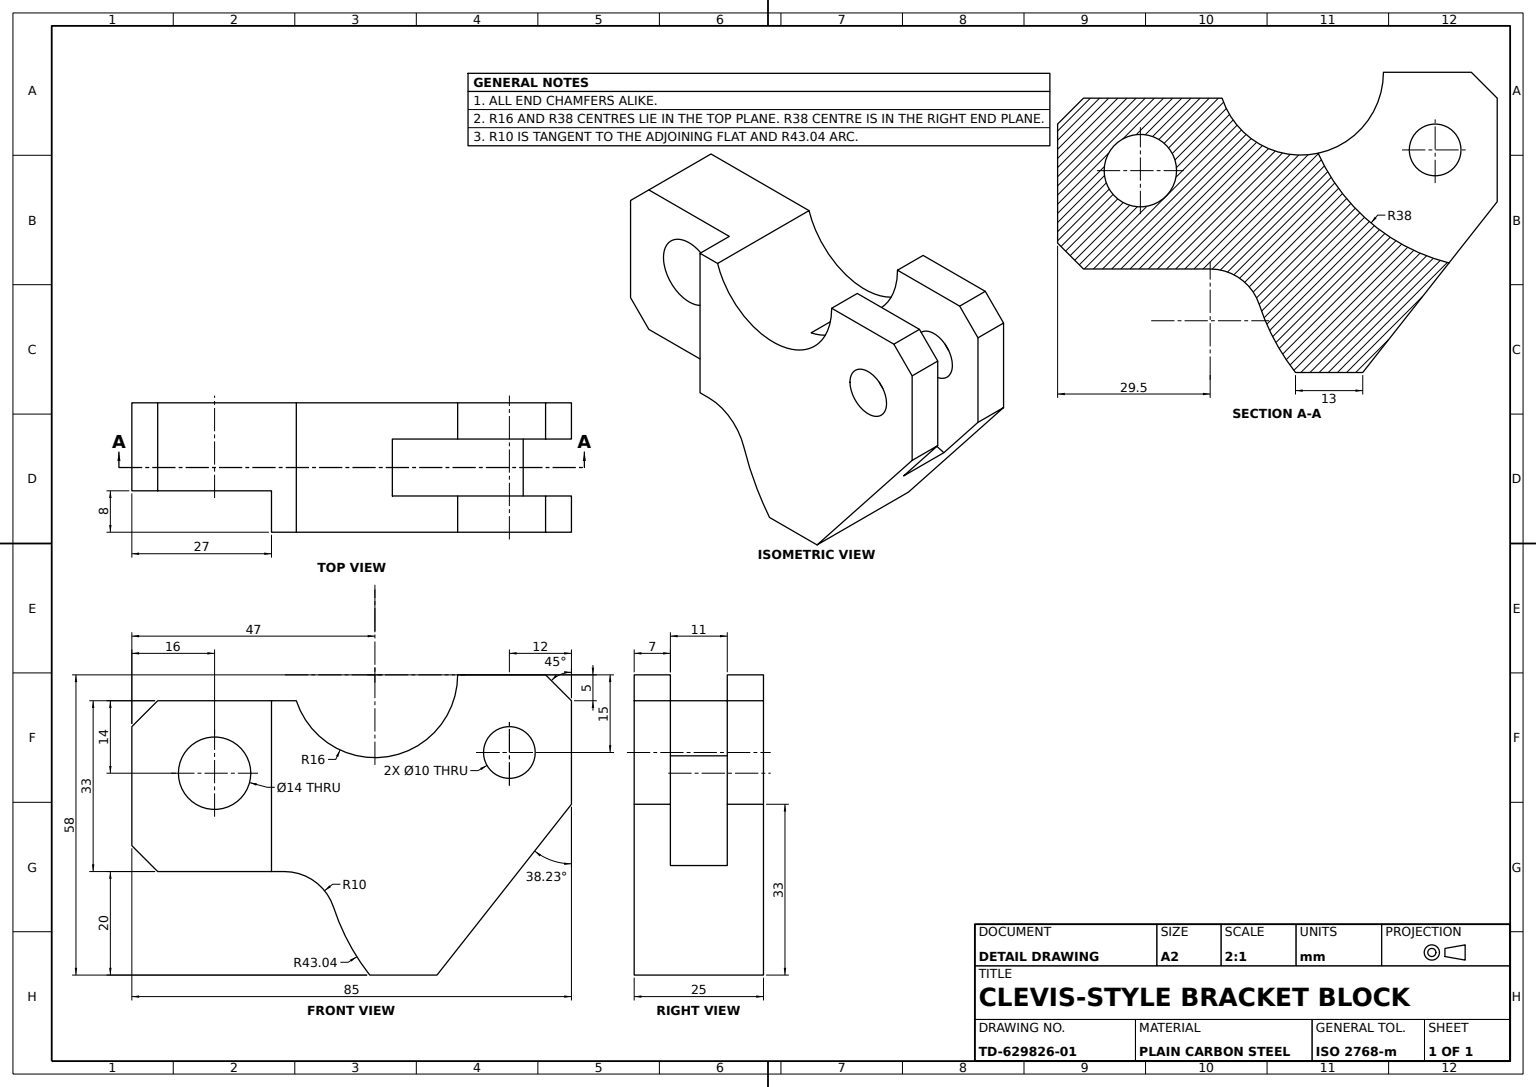
SolidWorks part; units mm, degrees
material "Plain Carbon Steel"
ref_plane "Front Plane" through (0, 0, 0) normal (0, 0, 1) x (1, 0, 0)
ref_plane "Top Plane" through (0, 0, 0) normal (0, 1, 0) x (1, 0, 0)
ref_plane "Right Plane" through (0, 0, 0) normal (1, 0, 0) x (0, 0, -1)
sketch "Bracket Profile Sketch" plane through (0, 0, 0) normal (0, 0, 1) x (1, 0, 0)
  line L0 (16, -3.84) -> (38, -3.84)
  line L1 (38, -3.84) -> (38, -28.84)
  line L2 (38, -28.84) -> (12, -61.84)
  line L3 (12, -61.84) -> (-1, -61.84)
  line L4 (-15.1987, -8.84) -> (-47, -8.84)
  line L5 (-47, -8.84) -> (-47, -41.84)
  line L6 (-47, -41.84) -> (-17.5042, -41.84)
  arc A0 (-15.1987, -8.84) -> (16, -3.84) centre (0, -3.84) ccw
  arc A4 (-8.0018, -48.7248) -> (-1, -61.84) centre (32.8971, -35.3167) ccw
  arc A5 (-8.0018, -48.7248) -> (-17.5042, -41.84) centre (-17.5042, -51.84) ccw
  circle A6 centre (-31, -22.84) radius 7
  circle A7 centre (26, -18.84) radius 5
  point P10 (5.5, -61.84)
  dimension "D1" = 32
  dimension "D2" = 22
  dimension "D9" = 10
  dimension "D12" = 14
  dimension "D13" = 10
  dimension "D3" = 25
  dimension "D4" = 26
  dimension "D5" = 13
  dimension "D6" = 20
  dimension "D7" = 33
  dimension "D8" = 58
  dimension "D10" = 3.84
  dimension "D11" = 85
  dimension "D14" = 16
  dimension "D15" = 14
  dimension "D16" = 15
  dimension "D17" = 12
  dimension "D18" = 17.5042
extrude "Bracket Body 25mm" add sketch "Bracket Profile Sketch" along normal mid plane 25
chamfer "Edge Chamfer 5mm" distance 5 angle 45 3 edges at (-47, -8.84, 0) (-47, -41.84, 0) (38, -3.84, 0)
sketch "Slot Sketch" plane through (0, 0, 12.5) normal (0, 0, 1) x (1, 0, 0)
  line L0 (-47, -8.84) -> (-20, -8.84)
  line L5 (-42, -41.84) -> (-17.5042, -41.84) construction
  line L8 (-47, -8.84) -> (-47, -41.84)
  line L9 (-47, -41.84) -> (-20, -41.84)
  line L10 (-20, -8.84) -> (-20, -41.84)
  dimension "D1" = 27
  dimension "D2" = 33
  dimension "D3" = 47
extrude "Slot Cut 8mm" cut sketch "Slot Sketch" against normal blind 8
ref_plane "Cross Hole Plane" through (0, 0, 0) normal (0, 0, 1) x (1, 0, 0)
sketch "Cross Hole Sketch" plane through (0, 0, 0) normal (0, 0, 1) x (1, 0, 0)
  circle A0 centre (38, -3.84) radius 38
  dimension "D1" = 76
  dimension "D2" = 38
  dimension "D3" = 3.84
extrude "Cross Hole Cut" cut sketch "Cross Hole Sketch" against normal mid plane 11
